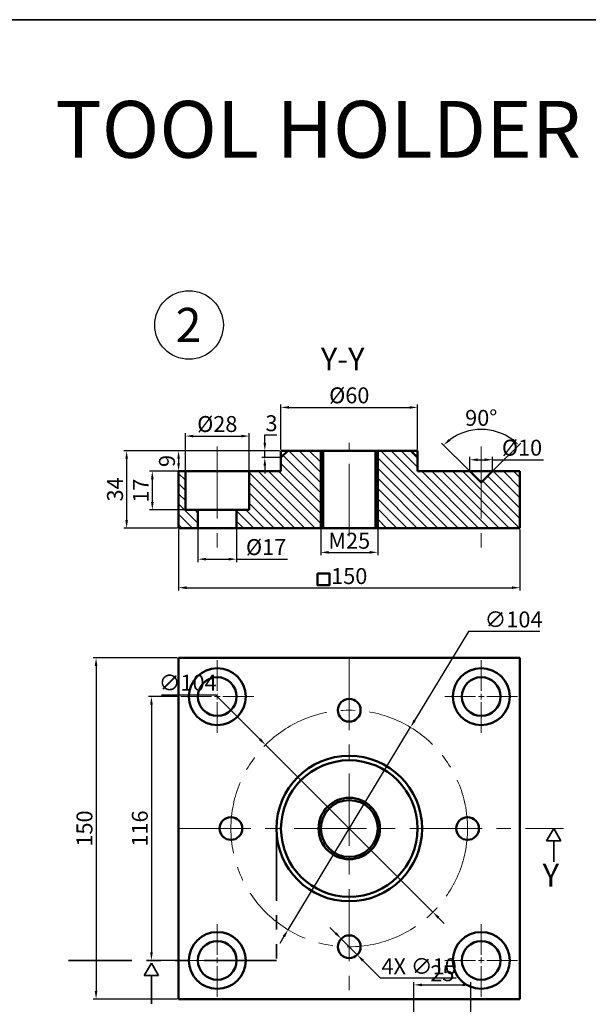
# Model space of a CAD drawing. Units: millimetres. Extents: x -5 to 1372, y -339 to 395.
# Tile 4 of 6: x 341 to 591, y -38 to 395. Entities that reach past the tile are written whole.
import ezdxf

# ---------------------------------------------------------------- set-up
doc = ezdxf.new("R2010")
doc.units = ezdxf.units.MM
doc.linetypes.add('CENTER', pattern=[50.8, 31.75, -6.35, 6.35, -6.35])
doc.linetypes.add('PHANTOM', pattern=[63.5, 31.75, -6.35, 6.35, -6.35, 6.35, -6.35])
for name, color, linetype, lineweight in [('M-CNTR', 1, 'CENTER', 18), ('M-DIMS', 2, 'Continuous', 25), ('M-HATC', 8, 'Continuous', 18), ('M-OUTL', 7, 'Continuous', 50), ('M-SECT', 4, 'PHANTOM', 35), ('M-TEXT', 3, 'Continuous', 25), ('M-TTLB', 7, 'Continuous', 35)]:
    doc.layers.add(name, color=color, linetype=linetype, lineweight=lineweight)
doc.styles.get("Standard").update_dxf_attribs({"font": 'arial.ttf'})
doc.dimstyles.new('ISO-25', dxfattribs={"dimtxt": 7, "dimasz": 3.5, "dimexe": 1.25, "dimexo": 0.625, "dimtad": 1, "dimtoh": 1, "dimtxsty": 'Standard', "dimcen": 2.5, "dimadec": 0, "dimazin": 0, "dimtfac": 1, "dimtmove": 0, "dimatfit": 3, "dimfxl": 1, "dimarcsym": 0})

# ---------------------------------------------------------------- blocks, each defined once
blk = doc.blocks.new('*U27')
at = {"layer": 'M-CNTR', "color": 0, "transparency": 16777216}
blk.add_line((0, 19.42), (0, -28.01), dxfattribs=at)
blk = doc.blocks.new('*U28')
at = {"layer": 'M-CNTR', "color": 0, "transparency": 16777216}
blk.add_line((0, -20.5), (0, 20.5), dxfattribs=at)
blk = doc.blocks.new('*U29')
at = {"layer": 'M-CNTR', "color": 0, "transparency": 16777216}
blk.add_line((0, 19.42), (0, -28.01), dxfattribs=at)
blk = doc.blocks.new('*D30')
at = {"layer": 'Defpoints', "color": 0, "transparency": 16777216}
for p in [(515.9, 224.26), (455.9, 205.2), (515.9, 205.2)]:
    blk.add_point(p, dxfattribs=at)
at = {"layer": 'M-DIMS', "color": 0, "lineweight": -2, "transparency": 16777216}
for p, q in [((455.9, 205.82), (455.9, 225.51)), ((515.9, 205.82), (515.9, 225.51)), ((459.4, 224.26), (512.4, 224.26))]:
    blk.add_line(p, q, dxfattribs=at)
at = {"layer": 'M-DIMS', "color": 0, "transparency": 16777216}
for points in [[(459.4, 224.85), (459.4, 223.68), (455.9, 224.26)], [(512.4, 224.85), (512.4, 223.68), (515.9, 224.26)]]:
    blk.add_solid(points, dxfattribs=at)
at = {"layer": 'M-DIMS', "color": 0, "transparency": 16777216, "insert": (485.9, 228.66), "char_height": 7, "attachment_point": 5}
blk.add_mtext('%%C60', dxfattribs=at)
blk = doc.blocks.new('*D31')
at = {"layer": 'Defpoints', "color": 0, "transparency": 16777216}
for p in [(455.9, 205.2), (448.8, 202.2), (455.9, 202.2)]:
    blk.add_point(p, dxfattribs=at)
at = {"layer": 'M-DIMS', "color": 0, "lineweight": -2, "transparency": 16777216}
for p, q in [((448.8, 208.7), (448.8, 212.2)), ((448.8, 212.2), (454.01, 212.2)), ((455.27, 205.2), (447.55, 205.2)), ((448.8, 202.2), (448.8, 205.2)), ((455.27, 202.2), (447.55, 202.2)), ((448.8, 198.7), (448.8, 195.2))]:
    blk.add_line(p, q, dxfattribs=at)
at = {"layer": 'M-DIMS', "color": 0, "transparency": 16777216}
for points in [[(448.22, 208.7), (449.38, 208.7), (448.8, 205.2)], [(448.22, 198.7), (449.38, 198.7), (448.8, 202.2)]]:
    blk.add_solid(points, dxfattribs=at)
at = {"layer": 'M-DIMS', "color": 0, "transparency": 16777216, "insert": (451.72, 216.4), "char_height": 7, "attachment_point": 5}
blk.add_mtext('3', dxfattribs=at)
blk = doc.blocks.new('*D32')
at = {"layer": 'Defpoints', "color": 0, "transparency": 16777216}
for p in [(441.9, 211.66), (413.9, 196.2), (441.9, 196.2)]:
    blk.add_point(p, dxfattribs=at)
at = {"layer": 'M-DIMS', "color": 0, "lineweight": -2, "transparency": 16777216}
for p, q in [((413.9, 196.82), (413.9, 212.91)), ((441.9, 196.82), (441.9, 212.91)), ((417.4, 211.66), (438.4, 211.66))]:
    blk.add_line(p, q, dxfattribs=at)
at = {"layer": 'M-DIMS', "color": 0, "transparency": 16777216}
for points in [[(417.4, 212.24), (417.4, 211.07), (413.9, 211.66)], [(438.4, 212.24), (438.4, 211.07), (441.9, 211.66)]]:
    blk.add_solid(points, dxfattribs=at)
at = {"layer": 'M-DIMS', "color": 0, "transparency": 16777216, "insert": (427.9, 216.05), "char_height": 7, "attachment_point": 5}
blk.add_mtext('%%C28', dxfattribs=at)
blk = doc.blocks.new('*D33')
at = {"layer": 'Defpoints', "color": 0, "transparency": 16777216}
for p in [(410.9, 196.2), (399.35, 179.2), (413.9, 179.2)]:
    blk.add_point(p, dxfattribs=at)
at = {"layer": 'M-DIMS', "color": 0, "lineweight": -2, "transparency": 16777216}
for p, q in [((410.27, 196.2), (398.1, 196.2)), ((399.35, 192.7), (399.35, 182.7)), ((413.27, 179.2), (398.1, 179.2))]:
    blk.add_line(p, q, dxfattribs=at)
at = {"layer": 'M-DIMS', "color": 0, "transparency": 16777216}
for points in [[(398.77, 192.7), (399.94, 192.7), (399.35, 196.2)], [(398.77, 182.7), (399.94, 182.7), (399.35, 179.2)]]:
    blk.add_solid(points, dxfattribs=at)
at = {"layer": 'M-DIMS', "color": 0, "transparency": 16777216, "insert": (395.21, 187.7), "char_height": 7, "attachment_point": 5, "rotation": 90}
blk.add_mtext('17', dxfattribs=at)
blk = doc.blocks.new('*D34')
at = {"layer": 'Defpoints', "color": 0, "transparency": 16777216}
for p in [(455.9, 205.2), (410.9, 196.2), (455.9, 196.2)]:
    blk.add_point(p, dxfattribs=at)
at = {"layer": 'M-DIMS', "color": 0, "lineweight": -2, "transparency": 16777216}
for p, q in [((455.27, 205.2), (409.65, 205.2)), ((410.9, 201.7), (410.9, 199.7)), ((455.27, 196.2), (409.65, 196.2))]:
    blk.add_line(p, q, dxfattribs=at)
at = {"layer": 'M-DIMS', "color": 0, "transparency": 16777216}
for points in [[(410.32, 201.7), (411.48, 201.7), (410.9, 205.2)], [(410.32, 199.7), (411.48, 199.7), (410.9, 196.2)]]:
    blk.add_solid(points, dxfattribs=at)
at = {"layer": 'M-DIMS', "color": 0, "transparency": 16777216, "insert": (406.7, 200.7), "char_height": 7, "attachment_point": 5, "rotation": 90}
blk.add_mtext('9', dxfattribs=at)
blk = doc.blocks.new('*D35')
at = {"layer": 'Defpoints', "color": 0, "transparency": 16777216}
for p in [(413.9, 205.2), (388.06, 171.2), (410.9, 171.2)]:
    blk.add_point(p, dxfattribs=at)
at = {"layer": 'M-DIMS', "color": 0, "lineweight": -2, "transparency": 16777216}
for p, q in [((413.27, 205.2), (386.81, 205.2)), ((388.06, 201.7), (388.06, 174.7)), ((410.27, 171.2), (386.81, 171.2))]:
    blk.add_line(p, q, dxfattribs=at)
at = {"layer": 'M-DIMS', "color": 0, "transparency": 16777216}
for points in [[(387.48, 201.7), (388.64, 201.7), (388.06, 205.2)], [(387.48, 174.7), (388.64, 174.7), (388.06, 171.2)]]:
    blk.add_solid(points, dxfattribs=at)
at = {"layer": 'M-DIMS', "color": 0, "transparency": 16777216, "insert": (383.86, 188.2), "char_height": 7, "attachment_point": 5, "rotation": 90}
blk.add_mtext('34', dxfattribs=at)
blk = doc.blocks.new('*D36')
at = {"layer": 'Defpoints', "color": 0, "transparency": 16777216}
for p in [(419.4, 171.2), (436.4, 171.2), (436.4, 157.54)]:
    blk.add_point(p, dxfattribs=at)
at = {"layer": 'M-DIMS', "color": 0, "lineweight": -2, "transparency": 16777216}
for p, q in [((419.4, 170.57), (419.4, 156.29)), ((436.4, 170.57), (436.4, 156.29)), ((422.9, 157.54), (432.9, 157.54)), ((436.4, 157.54), (458.79, 157.54))]:
    blk.add_line(p, q, dxfattribs=at)
at = {"layer": 'M-DIMS', "color": 0, "transparency": 16777216}
for points in [[(422.9, 158.12), (422.9, 156.96), (419.4, 157.54)], [(432.9, 158.12), (432.9, 156.96), (436.4, 157.54)]]:
    blk.add_solid(points, dxfattribs=at)
at = {"layer": 'M-DIMS', "color": 0, "transparency": 16777216, "insert": (449.35, 161.94), "char_height": 7, "attachment_point": 5}
blk.add_mtext('%%C17', dxfattribs=at)
blk = doc.blocks.new('*D37')
at = {"layer": 'Defpoints', "color": 0, "transparency": 16777216}
for p in [(473.4, 171.2), (498.4, 171.2), (498.4, 160.54)]:
    blk.add_point(p, dxfattribs=at)
at = {"layer": 'M-DIMS', "color": 0, "lineweight": -2, "transparency": 16777216}
for p, q in [((473.4, 170.57), (473.4, 159.29)), ((498.4, 170.57), (498.4, 159.29)), ((476.9, 160.54), (494.9, 160.54))]:
    blk.add_line(p, q, dxfattribs=at)
at = {"layer": 'M-DIMS', "color": 0, "transparency": 16777216}
for points in [[(476.9, 161.13), (476.9, 159.96), (473.4, 160.54)], [(494.9, 161.13), (494.9, 159.96), (498.4, 160.54)]]:
    blk.add_solid(points, dxfattribs=at)
at = {"layer": 'M-DIMS', "color": 0, "transparency": 16777216, "insert": (485.9, 164.74), "char_height": 7, "attachment_point": 5}
blk.add_mtext('M25', dxfattribs=at)
blk = doc.blocks.new('*D38')
at = {"layer": 'Defpoints', "color": 0, "transparency": 16777216}
for p in [(410.9, 171.2), (560.9, 171.2), (560.9, 144.99)]:
    blk.add_point(p, dxfattribs=at)
at = {"layer": 'M-DIMS', "color": 0, "lineweight": -2, "transparency": 16777216}
for p, q in [((410.9, 170.57), (410.9, 143.74)), ((560.9, 170.57), (560.9, 143.74)), ((414.4, 144.99), (557.4, 144.99))]:
    blk.add_line(p, q, dxfattribs=at)
at = {"layer": 'M-DIMS', "color": 0, "transparency": 16777216}
for points in [[(414.4, 145.58), (414.4, 144.41), (410.9, 144.99)], [(557.4, 145.58), (557.4, 144.41), (560.9, 144.99)]]:
    blk.add_solid(points, dxfattribs=at)
at = {"layer": 'M-DIMS', "color": 0, "transparency": 16777216, "insert": (485.9, 149.19), "char_height": 7, "attachment_point": 5}
blk.add_mtext('150', dxfattribs=at)
blk = doc.blocks.new('*D39')
at = {"layer": 'Defpoints', "color": 0, "transparency": 16777216}
for p in [(548.9, 201.26), (538.9, 196.2), (548.9, 196.2)]:
    blk.add_point(p, dxfattribs=at)
at = {"layer": 'M-DIMS', "color": 0, "lineweight": -2, "transparency": 16777216}
for p, q in [((538.9, 196.82), (538.9, 202.51)), ((542.4, 201.26), (545.4, 201.26)), ((548.9, 196.82), (548.9, 202.51)), ((548.9, 201.26), (571.27, 201.26))]:
    blk.add_line(p, q, dxfattribs=at)
at = {"layer": 'M-DIMS', "color": 0, "transparency": 16777216}
for points in [[(542.4, 201.84), (542.4, 200.67), (538.9, 201.26)], [(545.4, 201.84), (545.4, 200.67), (548.9, 201.26)]]:
    blk.add_solid(points, dxfattribs=at)
at = {"layer": 'M-DIMS', "color": 0, "transparency": 16777216, "insert": (561.83, 205.65), "char_height": 7, "attachment_point": 5}
blk.add_mtext('%%C10', dxfattribs=at)
blk = doc.blocks.new('*D40')
at = {"layer": 'Defpoints', "color": 0, "transparency": 16777216}
for p in [(549.94, 213.76), (538.9, 196.2), (548.9, 196.2), (543.9, 191.2), (543.9, 191.2)]:
    blk.add_point(p, dxfattribs=at)
at = {"layer": 'M-DIMS', "color": 0, "lineweight": -2, "transparency": 16777216}
for p, q in [((538.46, 196.64), (526.5, 208.6)), ((549.34, 196.64), (561.3, 208.6))]:
    blk.add_line(p, q, dxfattribs=at)
blk.add_arc((543.9, 191.2), 23.36, 53.5931, 126.4069, dxfattribs=at)
at = {"layer": 'M-DIMS', "color": 0, "transparency": 16777216}
for points in [[(530.42, 209.56), (529.65, 210.44), (527.38, 207.72)], [(558.14, 210.44), (557.38, 209.56), (560.42, 207.72)]]:
    blk.add_solid(points, dxfattribs=at)
at = {"layer": 'M-DIMS', "color": 0, "transparency": 16777216, "insert": (543.9, 218.76), "char_height": 7, "attachment_point": 5}
blk.add_mtext('90°', dxfattribs=at)
blk = doc.blocks.new('*U41')
at = {"layer": 'M-CNTR', "color": 0, "transparency": 16777216}
for p, q in [((0, 2.5), (0, 16)), ((-16, 0), (-2.5, 0)), ((2.5, 0), (16, 0)), ((0, -16), (0, -2.5))]:
    blk.add_line(p, q, dxfattribs=at)
at = {"layer": 'M-CNTR', "color": 0, "linetype": 'Continuous', "transparency": 16777216}
for p, q in [((-1.25, 0), (1.25, 0)), ((0, -1.25), (0, 1.25))]:
    blk.add_line(p, q, dxfattribs=at)
blk = doc.blocks.new('*U42')
at = {"layer": 'M-CNTR', "color": 0, "transparency": 16777216}
for p, q in [((0, 2.5), (0, 16)), ((-16, 0), (-2.5, 0)), ((2.5, 0), (16, 0)), ((0, -16), (0, -2.5))]:
    blk.add_line(p, q, dxfattribs=at)
at = {"layer": 'M-CNTR', "color": 0, "linetype": 'Continuous', "transparency": 16777216}
for p, q in [((-1.25, 0), (1.25, 0)), ((0, -1.25), (0, 1.25))]:
    blk.add_line(p, q, dxfattribs=at)
blk = doc.blocks.new('*U43')
at = {"layer": 'M-CNTR', "color": 0, "transparency": 16777216}
for p, q in [((0, 2.5), (0, 16)), ((-16, 0), (-2.5, 0)), ((2.5, 0), (16, 0)), ((0, -16), (0, -2.5))]:
    blk.add_line(p, q, dxfattribs=at)
at = {"layer": 'M-CNTR', "color": 0, "linetype": 'Continuous', "transparency": 16777216}
for p, q in [((-1.25, 0), (1.25, 0)), ((0, -1.25), (0, 1.25))]:
    blk.add_line(p, q, dxfattribs=at)
blk = doc.blocks.new('*U44')
at = {"layer": 'M-CNTR', "color": 0, "transparency": 16777216}
for p, q in [((0, 2.5), (0, 16)), ((-16, 0), (-2.5, 0)), ((2.5, 0), (16, 0)), ((0, -16), (0, -2.5))]:
    blk.add_line(p, q, dxfattribs=at)
at = {"layer": 'M-CNTR', "color": 0, "linetype": 'Continuous', "transparency": 16777216}
for p, q in [((-1.25, 0), (1.25, 0)), ((0, -1.25), (0, 1.25))]:
    blk.add_line(p, q, dxfattribs=at)
blk = doc.blocks.new('*D45')
at = {"layer": 'Defpoints', "color": 0, "transparency": 16777216}
for p in [(410.9, 114.12), (374.63, -35.88), (410.9, -35.88)]:
    blk.add_point(p, dxfattribs=at)
at = {"layer": 'M-DIMS', "color": 0, "lineweight": -2, "transparency": 16777216}
for p, q in [((410.27, 114.12), (373.38, 114.12)), ((374.63, 110.62), (374.63, -32.38)), ((410.27, -35.88), (373.38, -35.88))]:
    blk.add_line(p, q, dxfattribs=at)
at = {"layer": 'M-DIMS', "color": 0, "transparency": 16777216}
for points in [[(374.05, 110.62), (375.21, 110.62), (374.63, 114.12)], [(374.05, -32.38), (375.21, -32.38), (374.63, -35.88)]]:
    blk.add_solid(points, dxfattribs=at)
at = {"layer": 'M-DIMS', "color": 0, "transparency": 16777216, "insert": (370.43, 39.12), "char_height": 7, "attachment_point": 5, "rotation": 90}
blk.add_mtext('150', dxfattribs=at)
blk = doc.blocks.new('*D46')
at = {"layer": 'Defpoints', "color": 0, "transparency": 16777216}
for p in [(411.9, 97.12), (398.96, -18.88), (411.9, -18.88)]:
    blk.add_point(p, dxfattribs=at)
at = {"layer": 'M-DIMS', "color": 0, "lineweight": -2, "transparency": 16777216}
for p, q in [((411.27, 97.12), (397.71, 97.12)), ((398.96, 93.62), (398.96, -15.38)), ((411.27, -18.88), (397.71, -18.88))]:
    blk.add_line(p, q, dxfattribs=at)
at = {"layer": 'M-DIMS', "color": 0, "transparency": 16777216}
for points in [[(398.38, 93.62), (399.55, 93.62), (398.96, 97.12)], [(398.38, -15.38), (399.55, -15.38), (398.96, -18.88)]]:
    blk.add_solid(points, dxfattribs=at)
at = {"layer": 'M-DIMS', "color": 0, "transparency": 16777216, "insert": (394.76, 39.12), "char_height": 7, "attachment_point": 5, "rotation": 90}
blk.add_mtext('116', dxfattribs=at)
blk = doc.blocks.new('*D47')
at = {"layer": 'Defpoints', "color": 0, "transparency": 16777216}
for p in [(512.8, 83.62), (459, -5.39)]:
    blk.add_point(p, dxfattribs=at)
at = {"layer": 'M-DIMS', "color": 0, "lineweight": -2, "transparency": 16777216}
for p, q in [((538.25, 125.74), (514.61, 86.61)), ((569.63, 125.74), (538.25, 125.74)), ((459, -5.39), (512.8, 83.62)), ((457.19, -8.38), (455.38, -11.38))]:
    blk.add_line(p, q, dxfattribs=at)
at = {"layer": 'M-DIMS', "color": 0, "transparency": 16777216}
for points in [[(514.11, 86.92), (515.11, 86.31), (512.8, 83.62)], [(456.69, -8.08), (457.69, -8.68), (459, -5.39)]]:
    blk.add_solid(points, dxfattribs=at)
at = {"layer": 'M-DIMS', "color": 0, "transparency": 16777216, "insert": (558.11, 130.13), "char_height": 7, "attachment_point": 5}
blk.add_mtext('∅104', dxfattribs=at)
blk = doc.blocks.new('SECTION-ARROW')
for p, q in [((3.14, 5.44), (0, 0)), ((3.14, 5.44), (6.28, 0)), ((0, 0), (6.28, 0))]:
    blk.add_line(p, q)
blk = doc.blocks.new('*D96')
at = {"layer": 'Defpoints', "color": 0, "transparency": 16777216}
for p in [(539.31, -29.63), (514.31, -137.16), (539.31, -137.16)]:
    blk.add_point(p, dxfattribs=at)
at = {"layer": 'M-DIMS', "color": 0, "lineweight": -2, "transparency": 16777216}
for p, q in [((514.31, -136.53), (514.31, -28.38)), ((517.81, -29.63), (535.81, -29.63)), ((539.31, -136.53), (539.31, -28.38))]:
    blk.add_line(p, q, dxfattribs=at)
at = {"layer": 'M-DIMS', "color": 0, "transparency": 16777216}
for points in [[(517.81, -29.05), (517.81, -30.22), (514.31, -29.63)], [(535.81, -29.05), (535.81, -30.22), (539.31, -29.63)]]:
    blk.add_solid(points, dxfattribs=at)
at = {"layer": 'M-DIMS', "color": 0, "transparency": 16777216, "insert": (526.81, -25.43), "char_height": 7, "attachment_point": 5}
blk.add_mtext('25', dxfattribs=at)
blk = doc.blocks.new('*D98')
at = {"layer": 'Defpoints', "color": 0, "transparency": 16777216}
for p in [(449.12, 75.88), (522.68, 2.35)]:
    blk.add_point(p, dxfattribs=at)
at = {"layer": 'M-DIMS', "color": 0, "lineweight": -2, "transparency": 16777216}
for p, q in [((403.38, 97.94), (427.06, 97.94)), ((427.06, 97.94), (446.65, 78.35)), ((522.68, 2.35), (449.12, 75.88)), ((525.15, -0.12), (527.63, -2.6))]:
    blk.add_line(p, q, dxfattribs=at)
at = {"layer": 'M-DIMS', "color": 0, "transparency": 16777216}
for points in [[(447.06, 78.76), (446.23, 77.94), (449.12, 75.88)], [(525.56, 0.29), (524.74, -0.53), (522.68, 2.35)]]:
    blk.add_solid(points, dxfattribs=at)
at = {"layer": 'M-DIMS', "color": 0, "transparency": 16777216, "insert": (414.9, 102.33), "char_height": 7, "attachment_point": 5}
blk.add_mtext('∅104', dxfattribs=at)
blk = doc.blocks.new('*D99')
at = {"layer": 'Defpoints', "color": 0, "transparency": 16777216}
for p in [(482.37, -9.34), (489.43, -16.43)]:
    blk.add_point(p, dxfattribs=at)
at = {"layer": 'M-DIMS', "color": 0, "lineweight": -2, "transparency": 16777216}
for p, q in [((479.9, -6.86), (477.43, -4.38)), ((482.37, -9.34), (489.43, -16.43)), ((499.69, -26.73), (491.9, -18.91)), ((532.88, -26.73), (499.69, -26.73))]:
    blk.add_line(p, q, dxfattribs=at)
at = {"layer": 'M-DIMS', "color": 0, "transparency": 16777216}
for points in [[(480.31, -6.45), (479.49, -7.27), (482.37, -9.34)], [(492.31, -18.5), (491.48, -19.32), (489.43, -16.43)]]:
    blk.add_solid(points, dxfattribs=at)
at = {"layer": 'M-DIMS', "color": 0, "transparency": 16777216, "insert": (516.6, -22.33), "char_height": 7, "attachment_point": 5}
blk.add_mtext('4X ∅10', dxfattribs=at)

msp = doc.modelspace()

# ---------------------------------------------------------------- hatches: boundary and pattern name
at = {"layer": 'M-HATC'}
h = msp.add_hatch(dxfattribs=at)
h.set_pattern_fill('ANSI31', color=256, angle=90)
h.paths.add_polyline_path([(473.399, 205.198), (458.899, 205.198), (455.899, 202.198), (455.899, 196.198), (441.899, 196.198), (441.899, 179.198), (436.399, 179.198), (436.399, 171.198), (473.399, 171.198)])
h.paths.add_polyline_path([(543.899, 191.198), (538.899, 196.198), (515.899, 196.198), (515.899, 202.198), (512.899, 205.198), (498.399, 205.198), (498.399, 171.198), (543.899, 171.198)])
h.paths.add_polyline_path([(560.899, 196.198), (548.899, 196.198), (543.899, 191.198), (543.899, 171.198), (560.899, 171.198)])
h.paths.add_polyline_path([(419.399, 179.198), (413.899, 179.198), (413.899, 196.198), (410.899, 196.198), (410.899, 171.198), (419.399, 171.198)])

# ---------------------------------------------------------------- linework, layer by layer
at = {"layer": 'M-CNTR'}
for p, q in [((485.899, 114.115), (485.899, -35.885)), ((410.899, 39.115), (580.068, 39.115))]:
    msp.add_line(p, q, dxfattribs=at)
msp.add_circle((485.899, 39.115), 52, dxfattribs=at)
at = {"layer": 'M-OUTL'}
for p, q in [((515.899, 205.198), (455.899, 205.198)), ((455.899, 205.198), (455.899, 196.198)), ((458.899, 205.198), (455.899, 202.198)), ((473.399, 171.198), (473.399, 205.198)), ((474.399, 171.198), (474.399, 205.198)), ((497.399, 171.198), (497.399, 205.198)), ((498.399, 171.198), (498.399, 205.198)), ((512.899, 205.198), (515.899, 202.198)), ((515.899, 205.198), (515.899, 196.198)), ((410.899, 196.198), (410.899, 171.198)), ((410.899, 196.198), (455.899, 196.198)), ((413.899, 196.198), (413.899, 179.198)), ((441.899, 196.198), (441.899, 179.198)), ((515.899, 196.198), (560.899, 196.198)), ((538.899, 196.198), (543.899, 191.198)), ((548.899, 196.198), (543.899, 191.198)), ((560.899, 171.198), (560.899, 196.198)), ((413.899, 179.198), (441.899, 179.198)), ((419.399, 179.198), (419.399, 171.198)), ((436.399, 179.198), (436.399, 171.198)), ((410.899, 171.198), (560.899, 171.198)), ((410.899, 114.115), (560.899, 114.115)), ((410.899, -35.885), (410.899, 114.115)), ((560.899, 114.115), (560.899, -35.885)), ((560.899, -35.885), (410.899, -35.885))]:
    msp.add_line(p, q, dxfattribs=at)
msp.add_lwpolyline([(471.975, 151.254), (477.159, 151.254), (477.159, 146.071), (471.975, 146.071)], close=True, dxfattribs=at)
for centre, radius in [((427.899, 97.115), 12.5), ((543.899, 97.115), 12.5), ((427.899, 97.115), 8.5), ((543.899, 97.115), 8.5), ((485.899, 91.115), 5), ((485.899, 39.115), 32), ((485.899, 39.115), 30), ((485.899, 39.115), 13.5), ((485.899, 39.115), 12.5), ((433.899, 39.115), 5), ((537.899, 39.115), 5), ((427.899, -18.885), 12.5), ((485.899, -12.885), 5), ((543.899, -18.885), 12.5), ((427.899, -18.885), 8.5), ((543.899, -18.885), 8.5)]:
    msp.add_circle(centre, radius, dxfattribs=at)
at = {"layer": 'M-SECT'}
for p, q in [((453.899, 39.115), (453.899, -18.885)), ((575.781, 33.679), (575.781, 24.49)), ((453.899, -18.885), (362.528, -18.885)), ((398.962, -25.571), (398.962, -37.965))]:
    msp.add_line(p, q, dxfattribs=at)
at = {"layer": 'M-TEXT'}
msp.add_circle((415.481, 260.486), 15.085, dxfattribs=at)
at = {"layer": 'M-TTLB'}
msp.add_lwpolyline([(-4.944, 394.729), (1371.917, 394.729), (1371.917, -339.365), (-4.944, -339.365)], close=True, dxfattribs=at)

# ---------------------------------------------------------------- block references
at = {"layer": 'M-CNTR'}
for name, p in [('*U28', (485.899, 188.198)), ('*U27', (427.899, 187.698)), ('*U29', (543.899, 187.698)), ('*U41', (427.899, 97.115)), ('*U42', (543.899, 97.115)), ('*U44', (427.899, -18.885)), ('*U43', (543.899, -18.885))]:
    msp.add_blockref(name, p, dxfattribs=at)
at = {"layer": 'M-SECT', "rotation": 119.9999999999997}
for p in [(578.919, 33.679), (402.101, -25.571)]:
    msp.add_blockref('SECTION-ARROW', p, dxfattribs=at)

# ---------------------------------------------------------------- texts
at = {"layer": 'M-TEXT', "attachment_point": 1}
for s, width, insert, char_height in [('TOOL HOLDER', 274.88879, (356.707, 359.016), 25), ('2', 15, (409.586, 268.017), 15), ('Y-Y', 36.96755, (473.408, 250.557), 10), ('Y', 15.979, (570.858, 23.606), 10)]:
    msp.add_mtext_dynamic_manual_height_columns(s, width=width, gutter_width=12.5, heights=[0], dxfattribs=dict(at, insert=insert, char_height=char_height))

# ---------------------------------------------------------------- dimensions: what is measured, and where the dimension line sits
at = {"layer": 'M-DIMS'}
for base, p1, p2, text, picture, middle in [((515.899, 224.263), (455.899, 205.198), (515.899, 205.198), '%%C<>', '*D30', (485.899, 228.658)), ((441.899, 211.656), (413.899, 196.198), (441.899, 196.198), '%%C<>', '*D32', (427.899, 216.05)), ((548.899, 201.258), (538.899, 196.198), (548.899, 196.198), '%%C<>', '*D39', (561.833, 205.653)), ((436.399, 157.541), (419.399, 171.198), (436.399, 171.198), '%%C<>', '*D36', (449.345, 161.936)), ((498.399, 160.542), (473.399, 171.198), (498.399, 171.198), 'M<>', '*D37', (485.899, 164.741))]:
    dim = msp.add_linear_dim(base=base, p1=p1, p2=p2, text=text, dimstyle='ISO-25', override={"dimclrd": 0, "dimclre": 0, "dimclrt": 0}, dxfattribs=at)
    dim.commit()
    dim.dimension.update_dxf_attribs({"geometry": picture, "text_midpoint": middle})
for base, p1, p2, picture, middle in [((448.801, 202.198), (455.899, 205.198), (455.899, 202.198), '*D31', (451.718, 212.198)), ((388.061, 171.198), (413.899, 205.198), (410.899, 171.198), '*D35', (388.061, 188.198)), ((399.353, 179.198), (410.899, 196.198), (413.899, 179.198), '*D33', (399.353, 187.698))]:
    dim = msp.add_linear_dim(base=base, p1=p1, p2=p2, angle=90, dimstyle='ISO-25', override={"dimclrd": 0, "dimclre": 0, "dimclrt": 0}, dxfattribs=at)
    dim.commit()
    dim.dimension.update_dxf_attribs({"geometry": picture, "text_midpoint": middle, "dimtype": 160})
dim = msp.add_angular_dim_2l(base=(549.944, 213.761), line1=((538.899, 196.198), (543.899, 191.198)), line2=((548.899, 196.198), (543.899, 191.198)), dimstyle='ISO-25', override={"dimclrd": 0, "dimclre": 0, "dimclrt": 0}, dxfattribs=at)
dim.commit()
dim.dimension.update_dxf_attribs({"geometry": '*D40', "text_midpoint": (543.899, 218.756)})
for base, p1, p2, picture, middle in [((410.899, 196.198), (455.899, 205.198), (455.899, 196.198), '*D34', (406.7, 200.698)), ((374.629, -35.885), (410.899, 114.115), (410.899, -35.885), '*D45', (370.43, 39.115)), ((398.962, -18.885), (411.899, 97.115), (411.899, -18.885), '*D46', (394.763, 39.115))]:
    dim = msp.add_linear_dim(base=base, p1=p1, p2=p2, angle=90, dimstyle='ISO-25', override={"dimclrd": 0, "dimclre": 0, "dimclrt": 0}, dxfattribs=at)
    dim.commit()
    dim.dimension.update_dxf_attribs({"geometry": picture, "text_midpoint": middle})
for base, p1, p2, override, picture, middle in [((560.899, 144.993), (410.899, 171.198), (560.899, 171.198), {"dimclrd": 0, "dimclre": 0, "dimclrt": 0}, '*D38', (485.899, 149.192)), ((539.307, -29.633), (514.307, -137.159), (539.307, -137.159), {"dimdec": 0, "dimlfac": 1, "dimrnd": 0, "dimzin": 0, "dimdsep": 46, "dimlunit": 2}, '*D96', (526.807, -25.434))]:
    dim = msp.add_linear_dim(base=base, p1=p1, p2=p2, dimstyle='ISO-25', override=override, dxfattribs=at)
    dim.commit()
    dim.dimension.update_dxf_attribs({"geometry": picture, "text_midpoint": middle})
for p1, p2, override, picture, middle in [((459.001, -5.388), (512.796, 83.619), {"dimclrd": 0, "dimclre": 0, "dimclrt": 0}, '*D47', (558.105, 125.74)), ((522.675, 2.353), (449.122, 75.878), {"dimdec": 0, "dimlfac": 1, "dimrnd": 0, "dimzin": 0, "dimdsep": 46, "dimlunit": 2}, '*D98', (414.904, 97.936))]:
    dim = msp.add_diameter_dim_2p(p1=p1, p2=p2, dimstyle='ISO-25', override=override, dxfattribs=at)
    dim.commit()
    dim.dimension.update_dxf_attribs({"geometry": picture, "text_midpoint": middle, "dimtype": 163})
dim = msp.add_diameter_dim_2p(p1=(482.37, -9.342), p2=(489.427, -16.427), text='4X <>', dimstyle='ISO-25', override={"dimdec": 0, "dimlfac": 1, "dimrnd": 0, "dimzin": 0, "dimdsep": 46, "dimlunit": 2}, dxfattribs=at)
dim.commit()
dim.dimension.update_dxf_attribs({"geometry": '*D99', "text_midpoint": (516.597, -26.729)})

doc.saveas('drawing.dxf')
